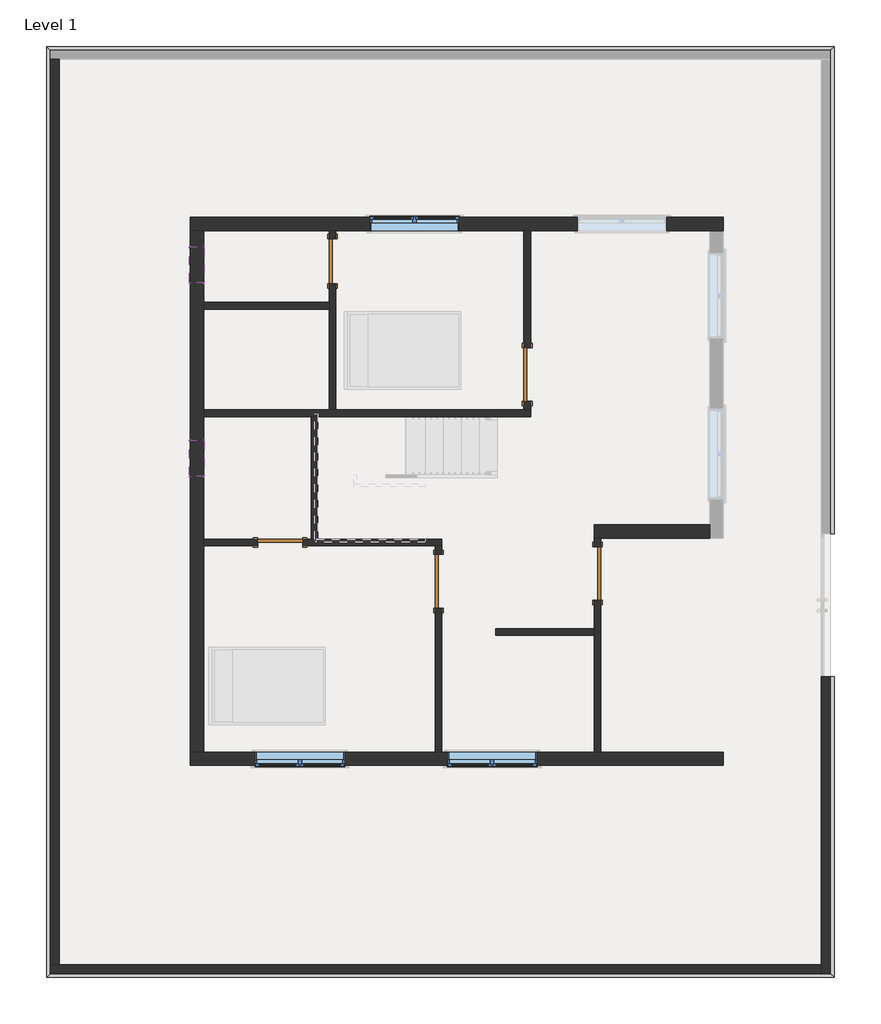
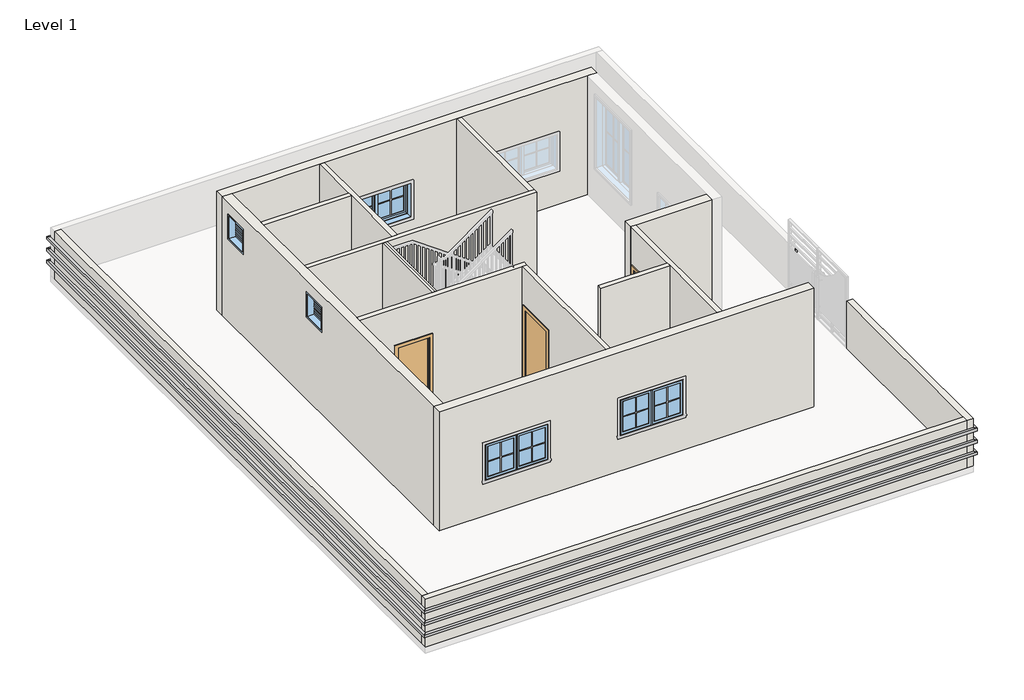
# One storey, part 1 of 3: 16 walls, 5 doors, 5 windows, 3 proxies.
"""IFC4 building model written with IfcOpenShell, lengths in millimetres."""

from ifc_helpers import new_model, si_unit, frame, origin, origin_with_axes, place, context, project, spatial, polyline, outline, extrude, faceted_brep, transform, mapped, element, save
from components import single_flush_3_17d80c48, single_flush_3_5e62189b, door_d8f5dbb5, window_c1d95f0f, window_f2d8fef0

model = new_model("IFC4")

# Units and contexts
model_context = context("Model", 3, world=origin())
ifc_project = project(units=[si_unit("LENGTHUNIT", "METRE", prefix="MILLI")], contexts=[model_context])

# Site, building, storey
site = spatial("IfcSite", under=ifc_project)
building = spatial("IfcBuilding", under=site)
storey = spatial("IfcBuildingStorey", under=building, Name="Level 1", Elevation=0.0)

# Proxies
placement = place(None, origin())
element("IfcBuildingElementProxy", 1, Name="Reveal", ObjectType="Reveal", at=placement, inside=storey, context=model_context, shape_type="SweptSolid", body=[
    extrude(outline(polyline([(5069.185534, 6860.1791885), (5161.260534, 6952.2541885), (5161.260534, -1330.2042021), (5069.185534, -1330.2042021), (5069.185534, 6860.1791885)])), frame((0.0, 0.0, 304.8), z_axis=(0.0, 0.0, 1.0), x_axis=(1.0, 0.0, 0.0)), (0.0, 0.0, 1.0), 67.7333333),
    extrude(outline(polyline([(-8138.814466, 6860.1791885), (-8230.889466, 6952.2541885), (5161.260534, 6952.2541885), (5069.185534, 6860.1791885), (-8138.814466, 6860.1791885)])), frame((0.0, 0.0, 304.8), z_axis=(0.0, 0.0, 1.0), x_axis=(1.0, 0.0, 0.0)), (0.0, 0.0, 1.0), 67.7333333),
    extrude(outline(polyline([(-8138.814466, -8786.2208115), (-8230.889466, -8878.2958115), (-8230.889466, 6952.2541885), (-8138.814466, 6860.1791885), (-8138.814466, -8786.2208115)])), frame((0.0, 0.0, 304.8), z_axis=(0.0, 0.0, 1.0), x_axis=(1.0, 0.0, 0.0)), (0.0, 0.0, 1.0), 67.7333333),
    extrude(outline(polyline([(5069.185534, -8786.2208115), (5161.260534, -8878.2958115), (-8230.889466, -8878.2958115), (-8138.814466, -8786.2208115), (5069.185534, -8786.2208115)])), frame((0.0, 0.0, 304.8), z_axis=(0.0, 0.0, 1.0), x_axis=(1.0, 0.0, 0.0)), (0.0, 0.0, 1.0), 67.7333333),
    extrude(outline(polyline([(5069.185534, -3768.6042021), (5161.260534, -3768.6042021), (5161.260534, -8878.2958115), (5069.185534, -8786.2208115), (5069.185534, -3768.6042021)])), frame((0.0, 0.0, 304.8), z_axis=(0.0, 0.0, 1.0), x_axis=(1.0, 0.0, 0.0)), (0.0, 0.0, 1.0), 67.7333333),
])
element("IfcBuildingElementProxy", 2, Name="Reveal", ObjectType="Reveal", at=placement, inside=storey, context=model_context, shape_type="SweptSolid", body=[
    extrude(outline(polyline([(5069.185534, 6860.1791885), (5161.260534, 6952.2541885), (5161.260534, -1330.2042021), (5069.185534, -1330.2042021), (5069.185534, 6860.1791885)])), frame((0.0, 0.0, 609.6), z_axis=(0.0, 0.0, 1.0), x_axis=(1.0, 0.0, 0.0)), (0.0, 0.0, 1.0), 67.7333333),
    extrude(outline(polyline([(-8138.814466, 6860.1791885), (-8230.889466, 6952.2541885), (5161.260534, 6952.2541885), (5069.185534, 6860.1791885), (-8138.814466, 6860.1791885)])), frame((0.0, 0.0, 609.6), z_axis=(0.0, 0.0, 1.0), x_axis=(1.0, 0.0, 0.0)), (0.0, 0.0, 1.0), 67.7333333),
    extrude(outline(polyline([(-8138.814466, -8786.2208115), (-8230.889466, -8878.2958115), (-8230.889466, 6952.2541885), (-8138.814466, 6860.1791885), (-8138.814466, -8786.2208115)])), frame((0.0, 0.0, 609.6), z_axis=(0.0, 0.0, 1.0), x_axis=(1.0, 0.0, 0.0)), (0.0, 0.0, 1.0), 67.7333333),
    extrude(outline(polyline([(5069.185534, -8786.2208115), (5161.260534, -8878.2958115), (-8230.889466, -8878.2958115), (-8138.814466, -8786.2208115), (5069.185534, -8786.2208115)])), frame((0.0, 0.0, 609.6), z_axis=(0.0, 0.0, 1.0), x_axis=(1.0, 0.0, 0.0)), (0.0, 0.0, 1.0), 67.7333333),
    extrude(outline(polyline([(5069.185534, -3768.6042021), (5161.260534, -3768.6042021), (5161.260534, -8878.2958115), (5069.185534, -8786.2208115), (5069.185534, -3768.6042021)])), frame((0.0, 0.0, 609.6), z_axis=(0.0, 0.0, 1.0), x_axis=(1.0, 0.0, 0.0)), (0.0, 0.0, 1.0), 67.7333333),
])
element("IfcBuildingElementProxy", 3, Name="Reveal", ObjectType="Reveal", at=placement, inside=storey, context=model_context, shape_type="SweptSolid", body=[
    extrude(outline(polyline([(5069.185534, 6860.1791885), (5161.260534, 6952.2541885), (5161.260534, -1330.2042021), (5069.185534, -1330.2042021), (5069.185534, 6860.1791885)])), frame((0.0, 0.0, 914.4), z_axis=(0.0, 0.0, 1.0), x_axis=(1.0, 0.0, 0.0)), (0.0, 0.0, 1.0), 67.7333333),
    extrude(outline(polyline([(-8138.814466, 6860.1791885), (-8230.889466, 6952.2541885), (5161.260534, 6952.2541885), (5069.185534, 6860.1791885), (-8138.814466, 6860.1791885)])), frame((0.0, 0.0, 914.4), z_axis=(0.0, 0.0, 1.0), x_axis=(1.0, 0.0, 0.0)), (0.0, 0.0, 1.0), 67.7333333),
    extrude(outline(polyline([(-8138.814466, -8786.2208115), (-8230.889466, -8878.2958115), (-8230.889466, 6952.2541885), (-8138.814466, 6860.1791885), (-8138.814466, -8786.2208115)])), frame((0.0, 0.0, 914.4), z_axis=(0.0, 0.0, 1.0), x_axis=(1.0, 0.0, 0.0)), (0.0, 0.0, 1.0), 67.7333333),
    extrude(outline(polyline([(5069.185534, -8786.2208115), (5161.260534, -8878.2958115), (-8230.889466, -8878.2958115), (-8138.814466, -8786.2208115), (5069.185534, -8786.2208115)])), frame((0.0, 0.0, 914.4), z_axis=(0.0, 0.0, 1.0), x_axis=(1.0, 0.0, 0.0)), (0.0, 0.0, 1.0), 67.7333333),
    extrude(outline(polyline([(5069.185534, -3768.6042021), (5161.260534, -3768.6042021), (5161.260534, -8878.2958115), (5069.185534, -8786.2208115), (5069.185534, -3768.6042021)])), frame((0.0, 0.0, 914.4), z_axis=(0.0, 0.0, 1.0), x_axis=(1.0, 0.0, 0.0)), (0.0, 0.0, 1.0), 67.7333333),
])

# Doors
single_flush_3_shape = single_flush_3_17d80c48(model_context)
element("IfcDoor", 4, ObjectType="Single-Flush : 3'", at=placement, inside=storey, context=model_context, shape_type="MappedRepresentation", body=[
    mapped(single_flush_3_shape, transform((-1566.5130704, -2143.0042021, 0.0), x_axis=(0.0, 1.0, 0.0), y_axis=(-1.0, 0.0, 0.0), z_axis=(0.0, 0.0, 1.0))),
])
single_flush_3_2_shape = single_flush_3_5e62189b(model_context)
element("IfcDoor", 5, ObjectType="Single-Flush : 3'", at=placement, inside=storey, context=model_context, shape_type="MappedRepresentation", body=[
    mapped(single_flush_3_2_shape, transform((1138.5869296, -2009.6542021, 0.0), x_axis=(0.0, 1.0, 0.0), y_axis=(-1.0, 0.0, 0.0), z_axis=(0.0, 0.0, 1.0))),
])
element("IfcDoor", 6, ObjectType="Single-Flush : 3'", at=placement, inside=storey, context=model_context, shape_type="MappedRepresentation", body=[
    mapped(single_flush_3_2_shape, transform((-55.2130704, 1374.8957979, 0.0), x_axis=(0.0, -1.0, 0.0), y_axis=(1.0, 0.0, 0.0), z_axis=(0.0, 0.0, 1.0))),
])
door_shape = door_d8f5dbb5(model_context)
element("IfcDoor", 7, ObjectType="Single-Flush : DOOR 2'6\"", at=placement, inside=storey, context=model_context, shape_type="MappedRepresentation", body=[
    mapped(door_shape, transform((-3369.9130704, 3298.9457979, 0.0), x_axis=(0.0, 1.0, 0.0), y_axis=(-1.0, 0.0, 0.0), z_axis=(0.0, 0.0, 1.0))),
])
element("IfcDoor", 8, ObjectType="Single-Flush : DOOR 2'6\"", at=placement, inside=storey, context=model_context, shape_type="MappedRepresentation", body=[
    mapped(door_shape, transform((-4258.9130704, -1482.6042021, 0.0), x_axis=(1.0, 0.0, 0.0), y_axis=(0.0, 1.0, 0.0), z_axis=(0.0, 0.0, 1.0))),
])

# Walls
element("IfcWall", 9, at=placement, inside=storey, context=model_context, shape_type="Brep", body=[
    faceted_brep([(4942.185534, -8659.2208115, 0.0), (-8011.814466, -8659.2208115, 0.0), (-8164.214466, -8659.2208115, 0.0), (-8164.214466, -8659.2208115, 304.8), (-8138.814466, -8659.2208115, 304.8), (-8138.814466, -8659.2208115, 372.5333333), (-8164.214466, -8659.2208115, 372.5333333), (-8164.214466, -8659.2208115, 609.6), (-8138.814466, -8659.2208115, 609.6), (-8138.814466, -8659.2208115, 677.3333333), (-8164.214466, -8659.2208115, 677.3333333), (-8164.214466, -8659.2208115, 914.4), (-8138.814466, -8659.2208115, 914.4), (-8138.814466, -8659.2208115, 982.1333333), (-8164.214466, -8659.2208115, 982.1333333), (-8164.214466, -8659.2208115, 1219.2), (-8011.814466, -8659.2208115, 1219.2), (4942.185534, -8659.2208115, 1219.2), (-8164.214466, -8811.6208115, 0.0), (4942.185534, -8811.6208115, 0.0), (4942.185534, -8811.6208115, 304.8), (-8164.214466, -8811.6208115, 304.8), (4942.185534, -8811.6208115, 1219.2), (-8164.214466, -8811.6208115, 1219.2), (-8164.214466, -8811.6208115, 982.1333333), (4942.185534, -8811.6208115, 982.1333333), (-8164.214466, -8811.6208115, 372.5333333), (4942.185534, -8811.6208115, 372.5333333), (4942.185534, -8811.6208115, 609.6), (-8164.214466, -8811.6208115, 609.6), (-8164.214466, -8811.6208115, 677.3333333), (4942.185534, -8811.6208115, 677.3333333), (4942.185534, -8811.6208115, 914.4), (-8164.214466, -8811.6208115, 914.4), (4942.185534, -8786.2208115, 982.1333333), (4942.185534, -8786.2208115, 914.4), (4942.185534, -8786.2208115, 677.3333333), (4942.185534, -8786.2208115, 609.6), (4942.185534, -8786.2208115, 372.5333333), (4942.185534, -8786.2208115, 304.8), (-8138.814466, -8786.2208115, 372.5333333), (-8138.814466, -8786.2208115, 304.8), (-8138.814466, -8786.2208115, 677.3333333), (-8138.814466, -8786.2208115, 609.6), (-8138.814466, -8786.2208115, 982.1333333), (-8138.814466, -8786.2208115, 914.4)], [[[0, 1, 2, 3, 4, 5, 6, 7, 8, 9, 10, 11, 12, 13, 14, 15, 16, 17]], [[18, 19, 20, 21]], [[22, 23, 24, 25]], [[26, 27, 28, 29]], [[30, 31, 32, 33]], [[2, 1, 0, 19, 18]], [[17, 16, 15, 23, 22]], [[0, 17, 22, 25, 34, 35, 32, 31, 36, 37, 28, 27, 38, 39, 20, 19]], [[2, 18, 21, 3]], [[23, 15, 14, 24]], [[6, 26, 29, 7]], [[10, 30, 33, 11]], [[40, 41, 39, 38]], [[41, 40, 5, 4]], [[5, 40, 38, 27, 26, 6]], [[39, 41, 4, 3, 21, 20]], [[9, 42, 36, 31, 30, 10]], [[37, 43, 8, 7, 29, 28]], [[42, 43, 37, 36]], [[43, 42, 9, 8]], [[13, 44, 34, 25, 24, 14]], [[35, 45, 12, 11, 33, 32]], [[44, 45, 35, 34]], [[45, 44, 13, 12]]]),
])
element("IfcWall", 10, at=placement, inside=storey, context=model_context, shape_type="SweptSolid", body=[
    extrude(outline(polyline([(0.0, -8011.814466), (1219.2, -8011.814466), (1219.2, -8164.214466), (982.1333333, -8164.214466), (982.1333333, -8138.814466), (914.4, -8138.814466), (914.4, -8164.214466), (677.3333333, -8164.214466), (677.3333333, -8138.814466), (609.6, -8138.814466), (609.6, -8164.214466), (372.5333333, -8164.214466), (372.5333333, -8138.814466), (304.8, -8138.814466), (304.8, -8164.214466), (0.0, -8164.214466), (0.0, -8011.814466)])), frame((0.0, -8659.2208115, 0.0), z_axis=(0.0, 1.0, 0.0), x_axis=(0.0, 0.0, 1.0)), (0.0, 0.0, 1.0), 15392.4),
])
element("IfcWall", 11, at=placement, inside=storey, context=model_context, shape_type="Brep", body=[
    faceted_brep([(4942.185534, -3768.6042021, 0.0), (4942.185534, -8659.2208115, 0.0), (4942.185534, -8811.6208115, 0.0), (4942.185534, -8811.6208115, 304.8), (4942.185534, -8786.2208115, 304.8), (4942.185534, -8786.2208115, 372.5333333), (4942.185534, -8811.6208115, 372.5333333), (4942.185534, -8811.6208115, 609.6), (4942.185534, -8786.2208115, 609.6), (4942.185534, -8786.2208115, 677.3333333), (4942.185534, -8811.6208115, 677.3333333), (4942.185534, -8811.6208115, 914.4), (4942.185534, -8786.2208115, 914.4), (4942.185534, -8786.2208115, 982.1333333), (4942.185534, -8811.6208115, 982.1333333), (4942.185534, -8811.6208115, 1219.2), (4942.185534, -8659.2208115, 1219.2), (4942.185534, -3768.6042021, 1219.2), (5094.585534, -8811.6208115, 0.0), (5094.585534, -3768.6042021, 0.0), (5094.585534, -3768.6042021, 304.8), (5094.585534, -8811.6208115, 304.8), (5094.585534, -3768.6042021, 1219.2), (5094.585534, -8811.6208115, 1219.2), (5094.585534, -8811.6208115, 982.1333333), (5094.585534, -3768.6042021, 982.1333333), (5094.585534, -8811.6208115, 372.5333333), (5094.585534, -3768.6042021, 372.5333333), (5094.585534, -3768.6042021, 609.6), (5094.585534, -8811.6208115, 609.6), (5094.585534, -8811.6208115, 677.3333333), (5094.585534, -3768.6042021, 677.3333333), (5094.585534, -3768.6042021, 914.4), (5094.585534, -8811.6208115, 914.4), (5069.185534, -3768.6042021, 982.1333333), (5069.185534, -3768.6042021, 914.4), (5069.185534, -3768.6042021, 677.3333333), (5069.185534, -3768.6042021, 609.6), (5069.185534, -3768.6042021, 372.5333333), (5069.185534, -3768.6042021, 304.8), (5069.185534, -8786.2208115, 372.5333333), (5069.185534, -8786.2208115, 304.8), (5069.185534, -8786.2208115, 677.3333333), (5069.185534, -8786.2208115, 609.6), (5069.185534, -8786.2208115, 982.1333333), (5069.185534, -8786.2208115, 914.4)], [[[0, 1, 2, 3, 4, 5, 6, 7, 8, 9, 10, 11, 12, 13, 14, 15, 16, 17]], [[18, 19, 20, 21]], [[22, 23, 24, 25]], [[26, 27, 28, 29]], [[30, 31, 32, 33]], [[2, 1, 0, 19, 18]], [[17, 16, 15, 23, 22]], [[0, 17, 22, 25, 34, 35, 32, 31, 36, 37, 28, 27, 38, 39, 20, 19]], [[2, 18, 21, 3]], [[23, 15, 14, 24]], [[6, 26, 29, 7]], [[10, 30, 33, 11]], [[40, 38, 27, 26, 6, 5]], [[39, 41, 4, 3, 21, 20]], [[38, 40, 41, 39]], [[41, 40, 5, 4]], [[42, 36, 31, 30, 10, 9]], [[37, 43, 8, 7, 29, 28]], [[36, 42, 43, 37]], [[43, 42, 9, 8]], [[44, 34, 25, 24, 14, 13]], [[35, 45, 12, 11, 33, 32]], [[34, 44, 45, 35]], [[45, 44, 13, 12]]]),
])
element("IfcWall", 12, ObjectType="WALL 4.5\"", at=placement, inside=storey, context=model_context, shape_type="Brep", body=[
    faceted_brep([(-3427.0630704, 3819.6457979, 0.0), (-3427.0630704, 3679.9457979, 0.0), (-3427.0630704, 3679.9457979, 2032.0), (-3427.0630704, 2917.9457979, 2032.0), (-3427.0630704, 2917.9457979, 0.0), (-3427.0630704, 2600.4457979, 0.0), (-3427.0630704, 2486.1457979, 0.0), (-3427.0630704, 771.6457979, 0.0), (-3427.0630704, 771.6457979, 3048.0), (-3427.0630704, 2486.1457979, 3048.0), (-3427.0630704, 2600.4457979, 3048.0), (-3427.0630704, 3819.6457979, 3048.0), (-3312.7630704, 3679.9457979, 2032.0), (-3312.7630704, 3679.9457979, 0.0), (-3312.7630704, 3819.6457979, 0.0), (-3312.7630704, 3819.6457979, 3048.0), (-3312.7630704, 771.6457979, 3048.0), (-3312.7630704, 771.6457979, 0.0), (-3312.7630704, 2917.9457979, 0.0), (-3312.7630704, 2917.9457979, 2032.0)], [[[0, 1, 2, 3, 4, 5, 6, 7, 8, 9, 10, 11]], [[12, 13, 14, 15, 16, 17, 18, 19]], [[18, 17, 7, 6, 5, 4]], [[14, 13, 1, 0]], [[0, 11, 15, 14]], [[8, 7, 17, 16]], [[2, 1, 13, 12]], [[3, 2, 12, 19]], [[4, 3, 19, 18]], [[11, 10, 9, 8, 16, 15]]]),
])
element("IfcWall", 13, ObjectType="WALL 4.5\"", at=placement, inside=storey, context=model_context, shape_type="Brep", body=[
    faceted_brep([(-5560.6630704, 657.3457979, 0.0), (-3731.8630704, 657.3457979, 0.0), (-3617.5630704, 657.3457979, 0.0), (1.9369296, 657.3457979, 0.0), (1.9369296, 657.3457979, 3048.0), (-3617.5630704, 657.3457979, 3048.0), (-3731.8630704, 657.3457979, 3048.0), (-5560.6630704, 657.3457979, 3048.0), (-5560.6630704, 771.6457979, 0.0), (-5560.6630704, 771.6457979, 3048.0), (-3427.0630704, 771.6457979, 3048.0), (-3312.7630704, 771.6457979, 3048.0), (-112.3630704, 771.6457979, 3048.0), (1.9369296, 771.6457979, 3048.0), (1.9369296, 771.6457979, 0.0), (-112.3630704, 771.6457979, 0.0), (-3312.7630704, 771.6457979, 0.0), (-3427.0630704, 771.6457979, 0.0)], [[[0, 1, 2, 3, 4, 5, 6, 7]], [[8, 9, 10, 11, 12, 13, 14, 15, 16, 17]], [[3, 2, 1, 0, 8, 17, 16, 15, 14]], [[7, 6, 5, 4, 13, 12, 11, 10, 9]], [[0, 7, 9, 8]], [[4, 3, 14, 13]]]),
])
element("IfcWall", 14, ObjectType="WALL 4.5\"", at=placement, inside=storey, context=model_context, shape_type="SweptSolid", body=[
    extrude(outline(polyline([(917.6957979, 2032.0), (917.6957979, 0.0), (771.6457979, 0.0), (771.6457979, 3048.0), (3819.6457979, 3048.0), (3819.6457979, 0.0), (1832.0957979, 0.0), (1832.0957979, 2032.0), (917.6957979, 2032.0)])), frame((-112.3630704, 0.0, 0.0), z_axis=(1.0, 0.0, 0.0), x_axis=(0.0, 1.0, 0.0)), (0.0, 0.0, 1.0), 114.3),
])
element("IfcWall", 15, ObjectType="WALL 4.5\"", at=placement, inside=storey, context=model_context, shape_type="SweptSolid", body=[
    extrude(outline(polyline([(-3427.0630704, 2486.1457979), (-5560.6630704, 2486.1457979), (-5560.6630704, 2600.4457979), (-3427.0630704, 2600.4457979), (-3427.0630704, 2486.1457979)])), origin_with_axes(), (0.0, 0.0, 1.0), 3048.0),
])
element("IfcWall", 16, ObjectType="WALL 4.5\"", at=placement, inside=storey, context=model_context, shape_type="Brep", body=[
    faceted_brep([(-3877.9130704, -1539.7542021, 2032.0), (-3877.9130704, -1539.7542021, 0.0), (-1623.6630704, -1539.7542021, 0.0), (-1509.3630704, -1539.7542021, 0.0), (-1509.3630704, -1539.7542021, 3048.0), (-1623.6630704, -1539.7542021, 3048.0), (-5560.6630704, -1539.7542021, 3048.0), (-5560.6630704, -1539.7542021, 0.0), (-4639.9130704, -1539.7542021, 0.0), (-4639.9130704, -1539.7542021, 2032.0), (-1509.3630704, -1425.4542021, 0.0), (-3617.5630704, -1425.4542021, 0.0), (-3731.8630704, -1425.4542021, 0.0), (-3877.9130704, -1425.4542021, 0.0), (-3877.9130704, -1425.4542021, 2032.0), (-4639.9130704, -1425.4542021, 2032.0), (-4639.9130704, -1425.4542021, 0.0), (-5560.6630704, -1425.4542021, 0.0), (-5560.6630704, -1425.4542021, 3048.0), (-3731.8630704, -1425.4542021, 3048.0), (-3617.5630704, -1425.4542021, 3048.0), (-1509.3630704, -1425.4542021, 3048.0)], [[[0, 1, 2, 3, 4, 5, 6, 7, 8, 9]], [[10, 11, 12, 13, 14, 15, 16, 17, 18, 19, 20, 21]], [[8, 7, 17, 16]], [[3, 2, 1, 13, 12, 11, 10]], [[6, 5, 4, 21, 20, 19, 18]], [[7, 6, 18, 17]], [[4, 3, 10, 21]], [[14, 13, 1, 0]], [[15, 14, 0, 9]], [[16, 15, 9, 8]]]),
])
element("IfcWall", 17, ObjectType="WALL 4.5\"", at=placement, inside=storey, context=model_context, shape_type="SweptSolid", body=[
    extrude(outline(polyline([(-1539.7542021, 0.0), (-1685.8042021, 0.0), (-1685.8042021, 2032.0), (-2600.2042021, 2032.0), (-2600.2042021, 0.0), (-5044.9542021, 0.0), (-5044.9542021, 3048.0), (-1539.7542021, 3048.0), (-1539.7542021, 0.0)])), frame((-1623.6630704, 0.0, 0.0), z_axis=(1.0, 0.0, 0.0), x_axis=(0.0, 1.0, 0.0)), (0.0, 0.0, 1.0), 114.3),
])
element("IfcWall", 18, ObjectType="WALL 4.5\"", at=placement, inside=storey, context=model_context, shape_type="Brep", body=[
    faceted_brep([(1195.7369296, -1552.4542021, 2032.0), (1195.7369296, -1552.4542021, 0.0), (1195.7369296, -1412.7542021, 0.0), (1195.7369296, -1412.7542021, 3048.0), (1195.7369296, -5044.9542021, 3048.0), (1195.7369296, -5044.9542021, 0.0), (1195.7369296, -2466.8542021, 0.0), (1195.7369296, -2466.8542021, 2032.0), (1081.4369296, -1412.7542021, 0.0), (1081.4369296, -1552.4542021, 0.0), (1081.4369296, -1552.4542021, 2032.0), (1081.4369296, -2466.8542021, 2032.0), (1081.4369296, -2466.8542021, 0.0), (1081.4369296, -2948.9967683, 0.0), (1081.4369296, -3063.2967683, 0.0), (1081.4369296, -5044.9542021, 0.0), (1081.4369296, -5044.9542021, 3048.0), (1081.4369296, -3063.2967683, 3048.0), (1081.4369296, -2948.9967683, 3048.0), (1081.4369296, -1412.7542021, 3048.0)], [[[0, 1, 2, 3, 4, 5, 6, 7]], [[8, 9, 10, 11, 12, 13, 14, 15, 16, 17, 18, 19]], [[6, 5, 15, 14, 13, 12]], [[2, 1, 9, 8]], [[3, 2, 8, 19]], [[5, 4, 16, 15]], [[10, 9, 1, 0]], [[11, 10, 0, 7]], [[12, 11, 7, 6]], [[4, 3, 19, 18, 17, 16]]]),
])
element("IfcWall", 19, ObjectType="WALL 4.5\"", at=placement, inside=storey, context=model_context, shape_type="SweptSolid", body=[
    extrude(outline(polyline([(-594.9630704, -2948.9967683), (1081.4369296, -2948.9967683), (1081.4369296, -3063.2967683), (-594.9630704, -3063.2967683), (-594.9630704, -2948.9967683)])), origin_with_axes(), (0.0, 0.0, 1.0), 3048.0),
])
element("IfcWall", 20, ObjectType="WALL 4.5\"", at=placement, inside=storey, context=model_context, shape_type="SweptSolid", body=[
    extrude(outline(polyline([(3048.0, -3731.8630704), (0.0, -3731.8630704), (0.0, -3617.5630704), (3048.0, -3617.5630704), (3048.0, -3668.3630704), (3048.0, -3731.8630704)])), frame((0.0, -1425.4542021, 0.0), z_axis=(0.0, 1.0, 0.0), x_axis=(0.0, 0.0, 1.0)), (0.0, 0.0, 1.0), 2082.8),
])
element("IfcWall", 21, ObjectType="WALL 9\"", at=placement, inside=storey, context=model_context, shape_type="Brep", body=[
    faceted_brep([(-5789.2630704, 3819.6457979, 0.0), (-5560.6630704, 3819.6457979, 0.0), (-3427.0630704, 3819.6457979, 0.0), (-3312.7630704, 3819.6457979, 0.0), (-112.3630704, 3819.6457979, 0.0), (1.9369296, 3819.6457979, 0.0), (3049.9369296, 3819.6457979, 0.0), (3278.5369296, 3819.6457979, 0.0), (3278.5369296, 3819.6457979, 3048.0), (3049.9369296, 3819.6457979, 3048.0), (1.9369296, 3819.6457979, 3048.0), (-112.3630704, 3819.6457979, 3048.0), (-3312.7630704, 3819.6457979, 3048.0), (-3427.0630704, 3819.6457979, 3048.0), (-5560.6630704, 3819.6457979, 3048.0), (-5789.2630704, 3819.6457979, 3048.0), (2316.5119296, 3819.6457979, 1828.8), (2316.5119296, 3819.6457979, 914.4), (792.5119296, 3819.6457979, 914.4), (792.5119296, 3819.6457979, 1828.8), (-1210.9130704, 3819.6457979, 1828.8), (-1210.9130704, 3819.6457979, 914.4), (-2734.9130704, 3819.6457979, 914.4), (-2734.9130704, 3819.6457979, 1828.8), (-5789.2630704, 4048.2457979, 0.0), (-5789.2630704, 4048.2457979, 3048.0), (3278.5369296, 4048.2457979, 3048.0), (3278.5369296, 4048.2457979, 0.0), (2316.5119296, 4048.2457979, 1828.8), (792.5119296, 4048.2457979, 1828.8), (792.5119296, 4048.2457979, 914.4), (2316.5119296, 4048.2457979, 914.4), (-1210.9130704, 4048.2457979, 1828.8), (-2734.9130704, 4048.2457979, 1828.8), (-2734.9130704, 4048.2457979, 914.4), (-1210.9130704, 4048.2457979, 914.4)], [[[0, 1, 2, 3, 4, 5, 6, 7, 8, 9, 10, 11, 12, 13, 14, 15], [16, 17, 18, 19], [20, 21, 22, 23]], [[24, 25, 26, 27], [28, 29, 30, 31], [32, 33, 34, 35]], [[7, 6, 5, 4, 3, 2, 1, 0, 24, 27]], [[8, 7, 27, 26]], [[0, 15, 25, 24]], [[17, 16, 28, 31]], [[18, 17, 31, 30]], [[19, 18, 30, 29]], [[16, 19, 29, 28]], [[21, 20, 32, 35]], [[22, 21, 35, 34]], [[23, 22, 34, 33]], [[20, 23, 33, 32]], [[15, 14, 13, 12, 11, 10, 9, 8, 26, 25]]]),
])
element("IfcWall", 22, ObjectType="WALL 9\"", at=placement, inside=storey, context=model_context, shape_type="Brep", body=[
    faceted_brep([(3049.9369296, -1184.1542021, 0.0), (1081.4369296, -1184.1542021, 0.0), (1081.4369296, -1184.1542021, 3048.0), (3049.9369296, -1184.1542021, 3048.0), (3049.9369296, -1412.7542021, 0.0), (3049.9369296, -1412.7542021, 3048.0), (1195.7369296, -1412.7542021, 3048.0), (1081.4369296, -1412.7542021, 3048.0), (1081.4369296, -1412.7542021, 0.0), (1195.7369296, -1412.7542021, 0.0)], [[[0, 1, 2, 3]], [[4, 5, 6, 7, 8, 9]], [[1, 0, 4, 9, 8]], [[0, 3, 5, 4]], [[2, 1, 8, 7]], [[3, 2, 7, 6, 5]]]),
])
element("IfcWall", 23, ObjectType="WALL 9\"", at=placement, inside=storey, context=model_context, shape_type="Brep", body=[
    faceted_brep([(3278.5369296, -5044.9542021, 0.0), (1195.7369296, -5044.9542021, 0.0), (1081.4369296, -5044.9542021, 0.0), (-1509.3630704, -5044.9542021, 0.0), (-1623.6630704, -5044.9542021, 0.0), (-5560.6630704, -5044.9542021, 0.0), (-5789.2630704, -5044.9542021, 0.0), (-5789.2630704, -5044.9542021, 3048.0), (-5560.6630704, -5044.9542021, 3048.0), (-1623.6630704, -5044.9542021, 3048.0), (-1509.3630704, -5044.9542021, 3048.0), (1081.4369296, -5044.9542021, 3048.0), (1195.7369296, -5044.9542021, 3048.0), (3278.5369296, -5044.9542021, 3048.0), (-4684.3630704, -5044.9542021, 1828.8), (-4684.3630704, -5044.9542021, 914.4), (-3160.3630704, -5044.9542021, 914.4), (-3160.3630704, -5044.9542021, 1828.8), (-1414.1130704, -5044.9542021, 1828.8), (-1414.1130704, -5044.9542021, 914.4), (109.8869296, -5044.9542021, 914.4), (109.8869296, -5044.9542021, 1828.8), (3278.5369296, -5273.5542021, 0.0), (3278.5369296, -5273.5542021, 3048.0), (-5789.2630704, -5273.5542021, 3048.0), (-5789.2630704, -5273.5542021, 0.0), (-4684.3630704, -5273.5542021, 1828.8), (-3160.3630704, -5273.5542021, 1828.8), (-3160.3630704, -5273.5542021, 914.4), (-4684.3630704, -5273.5542021, 914.4), (-1414.1130704, -5273.5542021, 1828.8), (109.8869296, -5273.5542021, 1828.8), (109.8869296, -5273.5542021, 914.4), (-1414.1130704, -5273.5542021, 914.4)], [[[0, 1, 2, 3, 4, 5, 6, 7, 8, 9, 10, 11, 12, 13], [14, 15, 16, 17], [18, 19, 20, 21]], [[22, 23, 24, 25], [26, 27, 28, 29], [30, 31, 32, 33]], [[6, 5, 4, 3, 2, 1, 0, 22, 25]], [[0, 13, 23, 22]], [[7, 6, 25, 24]], [[15, 14, 26, 29]], [[16, 15, 29, 28]], [[17, 16, 28, 27]], [[14, 17, 27, 26]], [[19, 18, 30, 33]], [[20, 19, 33, 32]], [[21, 20, 32, 31]], [[18, 21, 31, 30]], [[13, 12, 11, 10, 9, 8, 7, 24, 23]]]),
])
element("IfcWall", 24, ObjectType="WALL 9\"", at=placement, inside=storey, context=model_context, shape_type="Brep", body=[
    faceted_brep([(-5560.6630704, -5044.9542021, 0.0), (-5560.6630704, -1539.7542021, 0.0), (-5560.6630704, -1425.4542021, 0.0), (-5560.6630704, 657.3457979, 0.0), (-5560.6630704, 771.6457979, 0.0), (-5560.6630704, 2486.1457979, 0.0), (-5560.6630704, 2600.4457979, 0.0), (-5560.6630704, 3819.6457979, 0.0), (-5560.6630704, 3819.6457979, 3048.0), (-5560.6630704, 2600.4457979, 3048.0), (-5560.6630704, 2486.1457979, 3048.0), (-5560.6630704, 771.6457979, 3048.0), (-5560.6630704, 657.3457979, 3048.0), (-5560.6630704, -1425.4542021, 3048.0), (-5560.6630704, -1539.7542021, 3048.0), (-5560.6630704, -5044.9542021, 3048.0), (-5560.6630704, 257.2957979, 2743.2), (-5560.6630704, 257.2957979, 2133.6), (-5560.6630704, -352.3042021, 2133.6), (-5560.6630704, -352.3042021, 2743.2), (-5560.6630704, 3543.4207979, 2743.2), (-5560.6630704, 3543.4207979, 2133.6), (-5560.6630704, 2933.8207979, 2133.6), (-5560.6630704, 2933.8207979, 2743.2), (-5789.2630704, -5044.9542021, 0.0), (-5789.2630704, -5044.9542021, 3048.0), (-5789.2630704, 3819.6457979, 3048.0), (-5789.2630704, 3819.6457979, 0.0), (-5789.2630704, 257.2957979, 2743.2), (-5789.2630704, -352.3042021, 2743.2), (-5789.2630704, -352.3042021, 2133.6), (-5789.2630704, 257.2957979, 2133.6), (-5789.2630704, 3543.4207979, 2743.2), (-5789.2630704, 2933.8207979, 2743.2), (-5789.2630704, 2933.8207979, 2133.6), (-5789.2630704, 3543.4207979, 2133.6)], [[[0, 1, 2, 3, 4, 5, 6, 7, 8, 9, 10, 11, 12, 13, 14, 15], [16, 17, 18, 19], [20, 21, 22, 23]], [[24, 25, 26, 27], [28, 29, 30, 31], [32, 33, 34, 35]], [[7, 6, 5, 4, 3, 2, 1, 0, 24, 27]], [[0, 15, 25, 24]], [[8, 7, 27, 26]], [[17, 16, 28, 31]], [[18, 17, 31, 30]], [[19, 18, 30, 29]], [[16, 19, 29, 28]], [[21, 20, 32, 35]], [[22, 21, 35, 34]], [[23, 22, 34, 33]], [[20, 23, 33, 32]], [[15, 14, 13, 12, 11, 10, 9, 8, 26, 25]]]),
])

# Windows
window_shape = window_c1d95f0f(model_context)
element("IfcWindow", 25, ObjectType="Window-Casement-Double : WINDOW 6\"", at=placement, inside=storey, context=model_context, shape_type="MappedRepresentation", body=[
    mapped(window_shape, transform((-3922.3630704, -5159.2542021, 0.0), x_axis=(-1.0, 0.0, 0.0), y_axis=(0.0, -1.0, 0.0), z_axis=(0.0, 0.0, 1.0))),
])
element("IfcWindow", 26, ObjectType="Window-Casement-Double : WINDOW 6\"", at=placement, inside=storey, context=model_context, shape_type="MappedRepresentation", body=[
    mapped(window_shape, transform((-652.1130704, -5159.2542021, 0.0), x_axis=(-1.0, 0.0, 0.0), y_axis=(0.0, -1.0, 0.0), z_axis=(0.0, 0.0, 1.0))),
])
element("IfcWindow", 27, ObjectType="Window-Casement-Double : WINDOW 6\"", at=placement, inside=storey, context=model_context, shape_type="MappedRepresentation", body=[
    mapped(window_shape, transform((-1972.9130704, 3933.9457979, 0.0), x_axis=(1.0, 0.0, 0.0), y_axis=(0.0, 1.0, 0.0), z_axis=(0.0, 0.0, 1.0))),
])
window_2_shape = window_f2d8fef0(model_context)
element("IfcWindow", 28, ObjectType="Window-Louvers : 24\" x 24\"", at=placement, inside=storey, context=model_context, shape_type="MappedRepresentation", body=[
    mapped(window_2_shape, transform((-5668.6130704, -47.5042021, 1219.2), x_axis=(0.0, -1.0, 0.0), y_axis=(1.0, 0.0, 0.0), z_axis=(0.0, 0.0, 1.0))),
])
element("IfcWindow", 29, ObjectType="Window-Louvers : 24\" x 24\"", at=placement, inside=storey, context=model_context, shape_type="MappedRepresentation", body=[
    mapped(window_2_shape, transform((-5668.6130704, 3238.6207979, 1219.2), x_axis=(0.0, -1.0, 0.0), y_axis=(1.0, 0.0, 0.0), z_axis=(0.0, 0.0, 1.0))),
])

save(model, "model.ifc")

# Revit data of these elements
# Type "Single-Flush : 3'"
#   Type Mark = "8"
#   Construction Type Id = "MDOOR"
#   Assembly Code = "C1020"
#   Analytic Construction = "Metal"
#   Thickness = 0' - 2"
#   Heat Transfer Coefficient (U) = 0.651978 BTU/(h·ft²·°F)
#   Height = 6' - 8"
#   Trim Projection Ext = 0' - 1"
#   Trim Projection Int = 0' - 1"
#   Trim Width = 0' - 3"
#   Width = 3' - 0"
#   Define Thermal Properties by = 1
#   Door Material = Door - Panel
#   Frame Material = Door - Frame
#   Visual Light Transmittance = 0
#   Solar Heat Gain Coefficient = 0
#   Function = (empty or 0)
#   Wall Closure = (empty or 0)
# Type "Single-Flush : DOOR 2'6\""
#   Type Mark = "9"
#   Construction Type Id = "MDOOR"
#   Assembly Code = "C1020"
#   Analytic Construction = "Metal"
#   Thickness = 0' - 2"
#   Heat Transfer Coefficient (U) = 0.651978 BTU/(h·ft²·°F)
#   Height = 6' - 8"
#   Trim Projection Ext = 0' - 1"
#   Trim Projection Int = 0' - 1"
#   Trim Width = 0' - 3"
#   Width = 2' - 6"
#   Define Thermal Properties by = 1
#   Door Material = Door - Panel
#   Frame Material = Door - Frame
#   Visual Light Transmittance = 0
#   Solar Heat Gain Coefficient = 0
#   Function = (empty or 0)
#   Wall Closure = (empty or 0)
# Type
#   Assembly Code = "B2010"
#   Layers, outside or top first: 0' - 6" "Brick, Soldier Course" (function 1)
# Type "WALL 4.5\""
#   Assembly Code = "B2010"
#   Layers, outside or top first: 0' - 4 1/2" no material (function 1)
# Type "WALL 9\""
#   Assembly Code = "B2010"
#   Layers, outside or top first: 0' - 9" no material (function 1)
# Type "Window-Casement-Double : WINDOW 6\""
#   Type Mark = "18"
#   Fire Rating = "0.5h"
#   Assembly Code = "B2020100"
#   Analytic Construction = "Double glazing - domestic"
#   Frame Extension [instance default] = 0' - 0 1/4"
#   Window Inset [instance default] = 0' - 0"
#   Wall Thickness [instance default] = 0' - 6"
#   Interior Wall Closure [instance default] = 0' - 2 1/4"
#   Half Width = 2' - 6"
#   Visual Light Transmittance = 0.81
#   Thermal Resistance (R) = 1.8146 (h·ft²·°F)/BTU
#   Solar Heat Gain Coefficient = 0.76
#   Rough Width = 5' - 0 1/2"
#   Rough Height = 3' - 0 1/2"
#   Height = 3' - 0"
#   Heat Transfer Coefficient (U) = 0.5511 BTU/(h·ft²·°F)
#   Exterior Wall Closure [instance default] = 0' - 1 1/4"
#   Extension Jamb [instance default] = 0' - 2 1/4"
#   Default Sill Height = 3' - 0"
#   Width = 5' - 0"
#   Muntin Visibility = yes
#   Interior Trim Visibility [instance default] = yes
#   Exterior Trim Visibility [instance default] = yes
#   Extension Jamb Visibility [instance default] = yes
#   Interior Trim Material = Wood - Stained
#   Muntin Pattern = Muntin Pattern_2x2 : Muntin Pattern_2x2
#   Interior Trim = Trim-Window-Interior-Flat : Picture Frame
#   Interior Frame Material = Wood - Stained
#   Glass Panel Material = Glass
#   Exterior Trim Material = Clad - White
#   Exterior Trim = Trim-Window-Exterior-Flat : with Sill
#   Exterior Frame Material = Clad - White
#   Wall Closure = (empty or 0)
# Type "Window-Louvers : 24\" x 24\""
#   Type Mark = "19"
#   Construction Type Id = "GSP4R"
#   Assembly Code = "B20"
#   Analytic Construction = "1/8 in Pilkington single glazing"
#   Visual Light Transmittance = 0.9
#   Thermal Resistance (R) = 1.53941 (h·ft²·°F)/BTU
#   Solar Heat Gain Coefficient = 0.78
#   Max Height = 1' - 11.74264"
#   Height = 2' - 0"
#   Heat Transfer Coefficient (U) = 0.6496 BTU/(h·ft²·°F)
#   Blade Width [instance default] = 1' - 10 1/2"
#   Blade Vertical Thickness = 0' - 0.35355"
#   Blade Thickness = 0' - 0 1/4"
#   Blade Spacing = 0' - 1 1/2"
#   Blade Height = 0' - 1.85355"
#   Blade Depth = 0' - 3"
#   Blade Angle = 45.00°
#   Default Sill Height = 3' - 0"
#   Trim Projection_Exterior = 0' - 0 1/2"
#   Trim Projection_Interior = 0' - 0 1/2"
#   Trim Width_Exterior = 0' - 1 1/2"
#   Trim Width_Interior = 0' - 1 1/2"
#   Width = 2' - 0"
#   Max Blade Count = 12
#   Define Thermal Properties by = 1
#   Blade Count = 12
#   Frame Material = Birch
#   Louver Material = Birch
#   Trim Exterior Material = Birch
#   Trim Interior Material = Birch
#   Wall Closure = (empty or 0)
# Elements 4, 5, 6 (IfcDoor, "Single-Flush : 3'")
#   Phase Created = New Construction
#   Materials on its faces: "Door - Frame", "Door - Panel"
# Elements 7, 8 (IfcDoor, "Single-Flush : DOOR 2'6\"")
#   Phase Created = New Construction
#   Materials on its faces: "Door - Frame", "Door - Panel"
# Elements 9, 10, 11 (IfcWall)
#   Top Offset = 0' - 0"
#   Base Offset = 0' - 0"
#   Unconnected Height = 4' - 0"
#   wall height = 4' - 0"
#   Phase Created = New Construction
#   Base Constraint = Level 1
#   Materials on its faces: "Brick, Soldier Course", "Parking Stripe", "Clad - White"
# Elements 12, 14, 15, 17 (IfcWall, "WALL 4.5\"")
#   Top Offset = 0' - 0"
#   Base Offset = 0' - 0"
#   Unconnected Height = 10' - 0"
#   wall height = 10' - 0"
#   Phase Created = New Construction
#   Base Constraint = Level 1
#   Materials on its faces: "Default Wall"
# Elements 13, 16, 18, 19, 20 (IfcWall, "WALL 4.5\"")
#   Top Offset = 0' - 0"
#   Base Offset = 0' - 0"
#   Unconnected Height = 10' - 0"
#   wall height = 10' - 0"
#   Phase Created = New Construction
#   Base Constraint = Level 1
#   Materials on its faces: "Default Wall", "Wood - Stained"
# Elements 21, 23, 24 (IfcWall, "WALL 9\"")
#   Top Offset = 0' - 0"
#   Base Offset = 0' - 0"
#   Unconnected Height = 10' - 0"
#   wall height = 10' - 0"
#   Phase Created = New Construction
#   Base Constraint = Level 1
#   Materials on its faces: "Default Wall", "Wood - Stained"
# Element 22 (IfcWall, "WALL 9\"")
#   Top Offset = 0' - 0"
#   Base Offset = 0' - 0"
#   Unconnected Height = 10' - 0"
#   wall height = 10' - 0"
#   Phase Created = New Construction
#   Base Constraint = Level 1
#   Materials on its faces: "Wood - Stained", "Default Wall"
# Element 25 (IfcWindow, "Window-Casement-Double : WINDOW 6\"")
#   Mark = "1"
#   Window Inset = 0' - 0"
#   Interior Wall Closure = 0' - 2 1/4"
#   Frame Extension = 0' - 0 1/4"
#   Exterior Wall Closure = 0' - 1 1/4"
#   Interior Trim Visibility = yes
#   Exterior Trim Visibility = yes
#   Phase Created = New Construction
#   Materials on its faces: "Wood - Stained", "Glass", "Clad - White"
# Element 26 (IfcWindow, "Window-Casement-Double : WINDOW 6\"")
#   Mark = "2"
#   Window Inset = 0' - 0"
#   Interior Wall Closure = 0' - 2 1/4"
#   Frame Extension = 0' - 0 1/4"
#   Exterior Wall Closure = 0' - 1 1/4"
#   Interior Trim Visibility = yes
#   Exterior Trim Visibility = yes
#   Phase Created = New Construction
#   Materials on its faces: "Wood - Stained", "Glass", "Clad - White"
# Element 27 (IfcWindow, "Window-Casement-Double : WINDOW 6\"")
#   Mark = "5"
#   Window Inset = 0' - 0"
#   Interior Wall Closure = 0' - 2 1/4"
#   Frame Extension = 0' - 0 1/4"
#   Exterior Wall Closure = 0' - 1 1/4"
#   Interior Trim Visibility = yes
#   Exterior Trim Visibility = yes
#   Phase Created = New Construction
#   Materials on its faces: "Wood - Stained", "Glass", "Clad - White"
# Element 28 (IfcWindow, "Window-Louvers : 24\" x 24\"")
#   Mark = "6"
#   Blade Width = 1' - 10 1/2"
#   Phase Created = New Construction
#   Materials on its faces: "Birch"
# Element 29 (IfcWindow, "Window-Louvers : 24\" x 24\"")
#   Mark = "7"
#   Blade Width = 1' - 10 1/2"
#   Phase Created = New Construction
#   Materials on its faces: "Birch"
# Materials
#   "Door - Panel": class "Wood", colour RGB 210 159 95, transparency 0, Cost = 0
#   "Door - Frame": colour RGB 118 70 51, transparency 0, Cost = 0
#   "Brick, Soldier Course": class "Masonry", colour RGB 170 98 104, transparency 0, Description = "Common brick soldier coursed", Cost = 0
#   "Wood - Stained": class "Wood", colour RGB 224 178 126, transparency 0, Cost = 0
#   "Glass": class "Glass", colour RGB 0 128 192, transparency 0.75, Description = "Soda Lime Glass", Cost = 0
#   "Clad - White": class "Wood", colour RGB 242 242 238, transparency 0, Cost = 0
#   "Birch": class "Wood", colour RGB 224 178 126, transparency 0, Description = "Betula Alleghaniensis", Cost = 0
#   "Parking Stripe": class "Paint", colour RGB 250 250 91, transparency 0, Cost = 0
#   "Default Wall": colour RGB 128 128 128, transparency 0, Cost = 0
